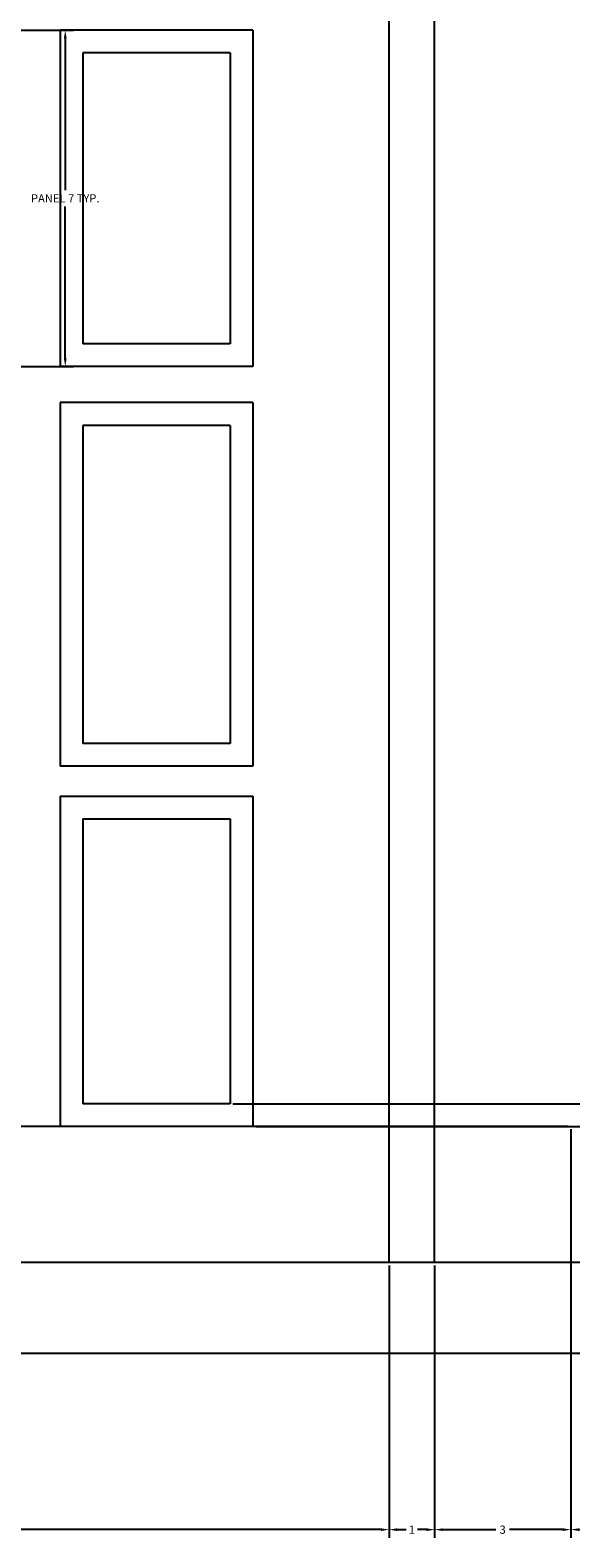
# Model space of a CAD drawing. Units: inches. Extents: x 12532.3 to 12594.9, y 6967.5 to 7063.
# Tile 2 of 9: x 12554.3 to 12566.2, y 6967.5 to 7000.7. Entities that reach past the tile are written whole.
import ezdxf

# ---------------------------------------------------------------- set-up
doc = ezdxf.new("R2010")
doc.units = ezdxf.units.IN
doc.header["$MEASUREMENT"] = 0
doc.header["$PDMODE"] = 98
doc.layers.add('A-ANNO-DIMS', color=2, linetype='Continuous', lineweight=18)
doc.layers.add('A-DOOR', color=4, linetype='Continuous', lineweight=25)
doc.styles.get("Standard").update_dxf_attribs({"font": 'arial.ttf'})
doc.dimstyles.get("Standard").update_dxf_attribs({"dimtxt": 0.18, "dimasz": 0.18, "dimexe": 0.18, "dimexo": 0.0625, "dimgap": 0.09, "dimtad": 0, "dimtih": 1, "dimtoh": 1, "dimdec": 4, "dimzin": 0, "dimdsep": 46, "dimtxsty": 'Standard', "dimcen": 0.09, "dimadec": 0, "dimazin": 0, "dimtfac": 1, "dimtdec": 4, "dimtofl": 0, "dimtmove": 0, "dimatfit": 3, "dimfxl": 1, "dimtolj": 1, "dimtzin": 0, "dimarcsym": 0})

# ---------------------------------------------------------------- blocks, each defined once
blk = doc.blocks.new('DOOR-PANEL-4_2x7_3')
for p, q in [((0, 7.273), (0, 0)), ((0, 7.273), (4.241, 7.273)), ((4.241, 7.273), (4.241, 0)), ((0.5, 6.773), (0.5, 0.5)), ((0.5, 6.773), (3.741, 6.773)), ((3.741, 6.773), (3.741, 0.5)), ((3.741, 0.5), (0.5, 0.5)), ((4.241, 0), (0, 0))]:
    blk.add_line(p, q)
blk = doc.blocks.new('DOOR-PANEL-4_2x7_4')
for p, q in [((4.241, 7.408), (0, 7.408)), ((0, 7.408), (0, 0)), ((4.241, 7.408), (4.241, 0)), ((3.741, 6.908), (0.5, 6.908)), ((0.5, 6.908), (0.5, 0.5)), ((3.741, 6.908), (3.741, 0.5)), ((3.741, 0.5), (0.5, 0.5)), ((4.241, 0), (0, 0))]:
    blk.add_line(p, q)
blk = doc.blocks.new('DOOR-PANEL-4_2x8_0')
for p, q in [((4.241, 8.003), (0, 8.003)), ((0, 8.003), (0, 0)), ((4.241, 8.003), (4.241, 0)), ((3.741, 7.503), (0.5, 7.503)), ((0.5, 7.503), (0.5, 0.5)), ((3.741, 7.503), (3.741, 0.5)), ((3.741, 0.5), (0.5, 0.5)), ((4.241, 0), (0, 0))]:
    blk.add_line(p, q)
blk = doc.blocks.new('*D25')
at = {"layer": 'A-ANNO-DIMS', "color": 0, "lineweight": -2, "transparency": 16777216}
for p, q in [((12553.994, 7000.738), (12555.223, 7000.738)), ((12555.043, 7000.558), (12555.043, 6997.214)), ((12555.043, 6993.51), (12555.043, 6996.854)), ((12553.994, 6993.33), (12555.223, 6993.33))]:
    blk.add_line(p, q, dxfattribs=at)
at = {"layer": 'A-ANNO-DIMS', "color": 0, "transparency": 16777216}
for points in [[(12555.013, 7000.558), (12555.073, 7000.558), (12555.043, 7000.738)], [(12555.013, 6993.51), (12555.073, 6993.51), (12555.043, 6993.33)]]:
    blk.add_solid(points, dxfattribs=at)
at = {"layer": 'Defpoints', "color": 0, "transparency": 16777216}
for p in [(12553.931, 7000.738), (12555.043, 7000.738), (12553.931, 6993.33)]:
    blk.add_point(p, dxfattribs=at)
at = {"layer": 'A-ANNO-DIMS', "color": 0, "transparency": 16777216, "insert": (12555.043, 6997.034), "char_height": 0.18, "attachment_point": 5}
blk.add_mtext('\\A1;PANEL 7 TYP.', dxfattribs=at)
blk = doc.blocks.new('*D35')
at = {"layer": 'A-ANNO-DIMS', "color": 0, "lineweight": -2, "transparency": 16777216}
for p, q in [((12542.45, 6973.534), (12542.45, 6967.537)), ((12562.172, 6973.534), (12562.172, 6967.537)), ((12542.63, 6967.717), (12551.927, 6967.717)), ((12561.992, 6967.717), (12552.695, 6967.717))]:
    blk.add_line(p, q, dxfattribs=at)
at = {"layer": 'A-ANNO-DIMS', "color": 0, "transparency": 16777216}
for points in [[(12542.63, 6967.747), (12542.63, 6967.687), (12542.45, 6967.717)], [(12561.992, 6967.747), (12561.992, 6967.687), (12562.172, 6967.717)]]:
    blk.add_solid(points, dxfattribs=at)
at = {"layer": 'Defpoints', "color": 0, "transparency": 16777216}
for p in [(12542.45, 6973.597), (12562.172, 6973.597), (12562.172, 6967.717)]:
    blk.add_point(p, dxfattribs=at)
at = {"layer": 'A-ANNO-DIMS', "color": 0, "transparency": 16777216, "insert": (12552.311, 6967.717), "char_height": 0.18, "attachment_point": 5}
blk.add_mtext('\\A1;19.72', dxfattribs=at)
blk = doc.blocks.new('*D36')
at = {"layer": 'A-ANNO-DIMS', "color": 0, "lineweight": -2, "transparency": 16777216}
for p, q in [((12562.172, 6973.534), (12562.172, 6967.537)), ((12563.172, 6973.534), (12563.172, 6967.537)), ((12562.352, 6967.717), (12562.549, 6967.717)), ((12562.992, 6967.717), (12562.795, 6967.717))]:
    blk.add_line(p, q, dxfattribs=at)
at = {"layer": 'A-ANNO-DIMS', "color": 0, "transparency": 16777216}
for points in [[(12562.352, 6967.747), (12562.352, 6967.687), (12562.172, 6967.717)], [(12562.992, 6967.747), (12562.992, 6967.687), (12563.172, 6967.717)]]:
    blk.add_solid(points, dxfattribs=at)
at = {"layer": 'Defpoints', "color": 0, "transparency": 16777216}
for p in [(12562.172, 6973.597), (12563.172, 6973.597), (12563.172, 6967.717)]:
    blk.add_point(p, dxfattribs=at)
at = {"layer": 'A-ANNO-DIMS', "color": 0, "transparency": 16777216, "insert": (12562.672, 6967.717), "char_height": 0.18, "attachment_point": 5}
blk.add_mtext('\\A1;1', dxfattribs=at)
blk = doc.blocks.new('*D37')
at = {"layer": 'A-ANNO-DIMS', "color": 0, "lineweight": -2, "transparency": 16777216}
for p, q in [((12566.172, 6976.534), (12566.172, 6967.537)), ((12563.172, 6973.534), (12563.172, 6967.537)), ((12563.352, 6967.717), (12564.523, 6967.717)), ((12565.992, 6967.717), (12564.821, 6967.717))]:
    blk.add_line(p, q, dxfattribs=at)
at = {"layer": 'A-ANNO-DIMS', "color": 0, "transparency": 16777216}
for points in [[(12563.352, 6967.747), (12563.352, 6967.687), (12563.172, 6967.717)], [(12565.992, 6967.747), (12565.992, 6967.687), (12566.172, 6967.717)]]:
    blk.add_solid(points, dxfattribs=at)
at = {"layer": 'Defpoints', "color": 0, "transparency": 16777216}
for p in [(12566.172, 6976.597), (12563.172, 6973.597), (12566.172, 6967.717)]:
    blk.add_point(p, dxfattribs=at)
at = {"layer": 'A-ANNO-DIMS', "color": 0, "transparency": 16777216, "insert": (12564.672, 6967.717), "char_height": 0.18, "attachment_point": 5}
blk.add_mtext('\\A1;3', dxfattribs=at)
blk = doc.blocks.new('*D38')
at = {"layer": 'A-ANNO-DIMS', "color": 0, "lineweight": -2, "transparency": 16777216}
for p, q in [((12566.172, 6976.534), (12566.172, 6967.537)), ((12579.894, 6976.534), (12579.894, 6967.537)), ((12566.352, 6967.717), (12572.579, 6967.717)), ((12579.714, 6967.717), (12573.487, 6967.717))]:
    blk.add_line(p, q, dxfattribs=at)
at = {"layer": 'A-ANNO-DIMS', "color": 0, "transparency": 16777216}
for points in [[(12566.352, 6967.747), (12566.352, 6967.687), (12566.172, 6967.717)], [(12579.714, 6967.747), (12579.714, 6967.687), (12579.894, 6967.717)]]:
    blk.add_solid(points, dxfattribs=at)
at = {"layer": 'Defpoints', "color": 0, "transparency": 16777216}
for p in [(12566.172, 6976.597), (12579.894, 6976.597), (12579.894, 6967.717)]:
    blk.add_point(p, dxfattribs=at)
at = {"layer": 'A-ANNO-DIMS', "color": 0, "transparency": 16777216, "insert": (12573.033, 6967.717), "char_height": 0.18, "attachment_point": 5}
blk.add_mtext('\\A1;13.722', dxfattribs=at)
blk = doc.blocks.new('*D43')
at = {"layer": 'A-ANNO-DIMS', "color": 0, "lineweight": -2, "transparency": 16777216}
for p, q in [((12566.11, 7015.929), (12532.39, 7015.929)), ((12532.57, 7015.749), (12532.57, 6996.445)), ((12532.57, 6976.777), (12532.57, 6996.081)), ((12566.11, 6976.597), (12532.39, 6976.597))]:
    blk.add_line(p, q, dxfattribs=at)
at = {"layer": 'A-ANNO-DIMS', "color": 0, "transparency": 16777216}
for points in [[(12532.54, 7015.749), (12532.6, 7015.749), (12532.57, 7015.929)], [(12532.54, 6976.777), (12532.6, 6976.777), (12532.57, 6976.597)]]:
    blk.add_solid(points, dxfattribs=at)
at = {"layer": 'Defpoints', "color": 0, "transparency": 16777216}
for p in [(12532.57, 7015.929), (12566.172, 7015.929), (12566.172, 6976.597)]:
    blk.add_point(p, dxfattribs=at)
at = {"layer": 'A-ANNO-DIMS', "color": 0, "transparency": 16777216, "insert": (12532.57, 6996.263), "char_height": 0.18, "attachment_point": 5}
blk.add_mtext('\\A1;39.33', dxfattribs=at)
blk = doc.blocks.new('*D61')
at = {"layer": 'A-ANNO-DIMS', "color": 0, "lineweight": -2, "transparency": 16777216}
for p, q in [((12592.773999, 6977.276753), (12592.773999, 6977.456753)), ((12558.734573, 6977.096753), (12592.953999, 6977.096753)), ((12559.234573, 6976.596753), (12592.953999, 6976.596753)), ((12592.773999, 6976.416753), (12592.773999, 6976.236753))]:
    blk.add_line(p, q, dxfattribs=at)
at = {"layer": 'A-ANNO-DIMS', "color": 0, "transparency": 16777216}
for points in [[(12592.743999, 6977.276753), (12592.803999, 6977.276753), (12592.773999, 6977.096753)], [(12592.743999, 6976.416753), (12592.803999, 6976.416753), (12592.773999, 6976.596753)]]:
    blk.add_solid(points, dxfattribs=at)
at = {"layer": 'Defpoints', "color": 0, "transparency": 16777216}
for p in [(12558.672073, 6977.096753), (12592.773999, 6977.096753), (12559.172073, 6976.596753)]:
    blk.add_point(p, dxfattribs=at)
at = {"layer": 'A-ANNO-DIMS', "color": 0, "transparency": 16777216, "insert": (12592.773999, 6976.846753), "char_height": 0.18, "attachment_point": 5}
blk.add_mtext('\\A1;0.5', dxfattribs=at)

msp = doc.modelspace()

# ---------------------------------------------------------------- linework, layer by layer
at = {"layer": 'A-DOOR'}
for p, q in [((12562.1721, 6973.5968), (12562.1721, 7018.9287)), ((12563.1721, 6973.5968), (12563.1721, 7018.9287))]:
    msp.add_line(p, q, dxfattribs=at)
msp.add_lwpolyline([(12536.4501, 7020.9287), (12588.894, 7020.9287), (12588.894, 6971.5968), (12536.4501, 6971.5968)], close=True, dxfattribs=at)
msp.add_lwpolyline([(12582.894, 6973.5968), (12542.4501, 6973.5968)], dxfattribs=at)

# ---------------------------------------------------------------- block references
for name, p in [('DOOR-PANEL-4_2x7_4', (12554.9313, 6993.33)), ('DOOR-PANEL-4_2x8_0', (12554.9313, 6984.532)), ('DOOR-PANEL-4_2x7_3', (12554.9313, 6976.597))]:
    msp.add_blockref(name, p, dxfattribs=at)

# ---------------------------------------------------------------- dimensions: what is measured, and where the dimension line sits
at = {"layer": 'A-ANNO-DIMS'}
for base, p1, p2, override, picture, middle in [((12532.5701, 7015.9287), (12566.1721, 6976.5968), (12566.1721, 7015.9287), {"dimdec": 2, "dimlfac": 1, "dimrnd": 0, "dimzin": 0, "dimdsep": 46, "dimlunit": 2}, '*D43', (12532.5701, 6996.2627)), ((12592.774, 6977.0968), (12559.1721, 6976.5968), (12558.6721, 6977.0968), {"dimdec": 1, "dimlfac": 1, "dimrnd": 0, "dimzin": 0, "dimdsep": 46, "dimlunit": 2}, '*D61', (12592.774, 6976.8468))]:
    dim = msp.add_linear_dim(base=base, p1=p1, p2=p2, angle=90, dimstyle='Standard', override=override, dxfattribs=at)
    dim.commit()
    dim.dimension.update_dxf_attribs({"geometry": picture, "text_midpoint": middle})
dim = msp.add_linear_dim(base=(12555.0425, 7000.7376), p1=(12553.9314, 6993.3303), p2=(12553.9314, 7000.7376), angle=90, text='PANEL <> TYP.', dimstyle='Standard', override={"dimdec": 0, "dimrnd": 0, "dimzin": 0, "dimlunit": 2}, dxfattribs=at)
dim.commit()
dim.dimension.update_dxf_attribs({"geometry": '*D25', "text_midpoint": (12555.0425, 6997.034)})
for base, p1, p2, override, picture, middle in [((12566.1721, 6967.7168), (12563.1721, 6973.5968), (12566.1721, 6976.5968), {"dimdec": 0, "dimlfac": 1, "dimrnd": 0, "dimzin": 0, "dimdsep": 46, "dimlunit": 2}, '*D37', (12564.6721, 6967.7168)), ((12579.894, 6967.7168), (12566.1721, 6976.5968), (12579.894, 6976.5968), {"dimdec": 3, "dimlfac": 1, "dimrnd": 0, "dimzin": 0, "dimdsep": 46, "dimlunit": 2}, '*D38', (12573.033, 6967.7168)), ((12562.1721, 6967.7168), (12542.4501, 6973.5968), (12562.1721, 6973.5968), {"dimdec": 2, "dimlfac": 1, "dimrnd": 0, "dimzin": 0, "dimdsep": 46, "dimlunit": 2}, '*D35', (12552.3111, 6967.7168)), ((12563.1721, 6967.7168), (12562.1721, 6973.5968), (12563.1721, 6973.5968), {"dimdec": 0, "dimlfac": 1, "dimrnd": 0, "dimzin": 0, "dimdsep": 46, "dimlunit": 2}, '*D36', (12562.6721, 6967.7168))]:
    dim = msp.add_linear_dim(base=base, p1=p1, p2=p2, dimstyle='Standard', override=override, dxfattribs=at)
    dim.commit()
    dim.dimension.update_dxf_attribs({"geometry": picture, "text_midpoint": middle})

doc.saveas('drawing.dxf')
